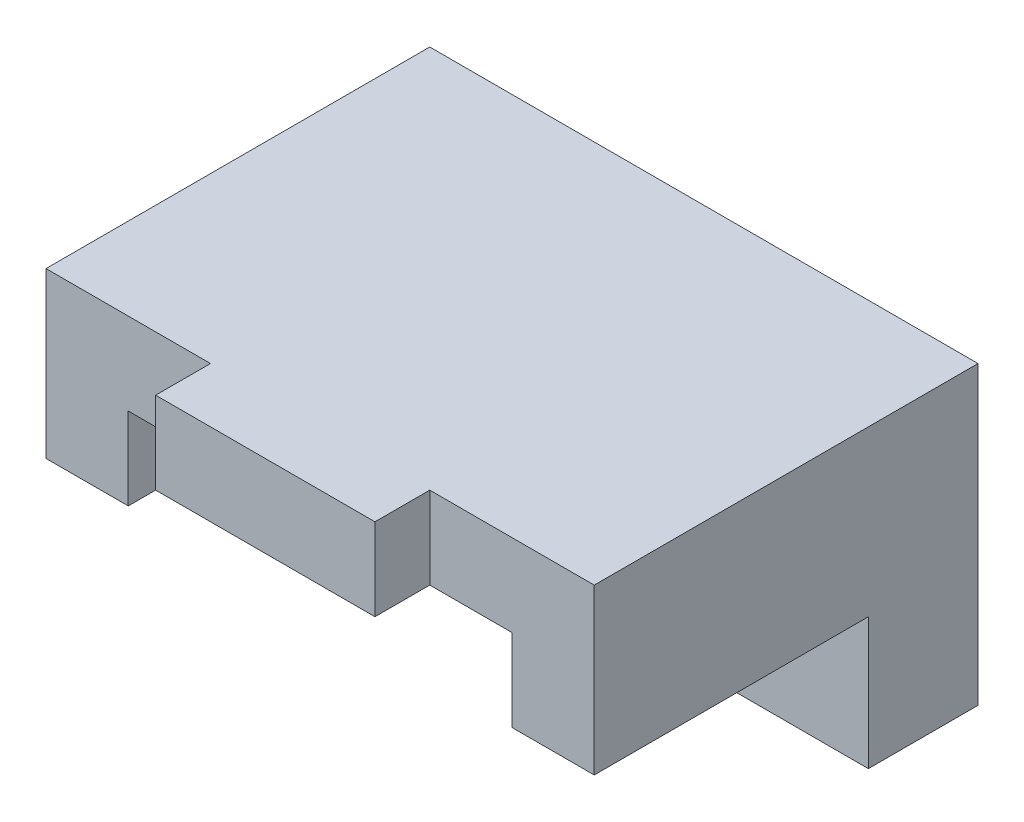
ISO-10303-21;
HEADER;
FILE_DESCRIPTION(('STEP AP214'),'2;1');
FILE_NAME('part.step','',(''),(''),'','','');
FILE_SCHEMA(('AUTOMOTIVE_DESIGN { 1 0 10303 214 1 1 1 1 }'));
ENDSEC;
DATA;
#1=APPLICATION_CONTEXT('core data for automotive mechanical design processes');
#2=APPLICATION_PROTOCOL_DEFINITION('international standard','automotive_design',2000,#1);
#3=PRODUCT_CONTEXT('',#1,'mechanical');
#4=PRODUCT('Part','Part','',(#3));
#5=PRODUCT_RELATED_PRODUCT_CATEGORY('part','',(#4));
#6=PRODUCT_DEFINITION_FORMATION('','',#4);
#7=PRODUCT_DEFINITION_CONTEXT('part definition',#1,'design');
#8=PRODUCT_DEFINITION('design','',#6,#7);
#9=PRODUCT_DEFINITION_SHAPE('','',#8);
#10=(LENGTH_UNIT() NAMED_UNIT(*) SI_UNIT(.MILLI.,.METRE.));
#11=(NAMED_UNIT(*) PLANE_ANGLE_UNIT() SI_UNIT($,.RADIAN.));
#12=(NAMED_UNIT(*) SI_UNIT($,.STERADIAN.) SOLID_ANGLE_UNIT());
#13=UNCERTAINTY_MEASURE_WITH_UNIT(LENGTH_MEASURE(1.E-05),#10,'distance_accuracy_value','');
#14=(GEOMETRIC_REPRESENTATION_CONTEXT(3) GLOBAL_UNCERTAINTY_ASSIGNED_CONTEXT((#13)) GLOBAL_UNIT_ASSIGNED_CONTEXT((#10,
#11,#12)) REPRESENTATION_CONTEXT('',''));
#15=CARTESIAN_POINT('',(0.,0.,0.));
#16=DIRECTION('',(0.,0.,1.));
#17=DIRECTION('',(1.,0.,0.));
#18=AXIS2_PLACEMENT_3D('',#15,#16,#17);
#19=CARTESIAN_POINT('',(0.,0.,200.));
#20=DIRECTION('',(0.,1.,0.));
#21=DIRECTION('',(0.,0.,1.));
#22=AXIS2_PLACEMENT_3D('',#19,#20,#21);
#23=PLANE('',#22);
#24=DIRECTION('',(0.,0.,1.));
#25=VECTOR('',#24,1.);
#26=CARTESIAN_POINT('',(750.,0.,50.));
#27=LINE('',#26,#25);
#28=CARTESIAN_POINT('',(750.,0.,50.));
#29=VERTEX_POINT('',#28);
#30=CARTESIAN_POINT('',(750.,0.,200.));
#31=VERTEX_POINT('',#30);
#32=EDGE_CURVE('E242',#29,#31,#27,.T.);
#33=ORIENTED_EDGE('',*,*,#32,.F.);
#34=DIRECTION('',(1.,0.,0.));
#35=VECTOR('',#34,1.);
#36=CARTESIAN_POINT('',(0.,0.,50.));
#37=LINE('',#36,#35);
#38=CARTESIAN_POINT('',(250.,0.,50.));
#39=VERTEX_POINT('',#38);
#40=EDGE_CURVE('E233',#39,#29,#37,.T.);
#41=ORIENTED_EDGE('',*,*,#40,.F.);
#42=DIRECTION('',(0.,0.,1.));
#43=VECTOR('',#42,1.);
#44=CARTESIAN_POINT('',(250.,0.,50.));
#45=LINE('',#44,#43);
#46=CARTESIAN_POINT('',(250.,0.,200.));
#47=VERTEX_POINT('',#46);
#48=EDGE_CURVE('E246',#39,#47,#45,.T.);
#49=ORIENTED_EDGE('',*,*,#48,.T.);
#50=DIRECTION('',(1.,0.,0.));
#51=VECTOR('',#50,1.);
#52=CARTESIAN_POINT('',(0.,0.,200.));
#53=LINE('',#52,#51);
#54=CARTESIAN_POINT('',(0.,0.,200.));
#55=VERTEX_POINT('',#54);
#56=EDGE_CURVE('E326',#55,#47,#53,.T.);
#57=ORIENTED_EDGE('',*,*,#56,.F.);
#58=DIRECTION('',(0.,0.,-1.));
#59=VECTOR('',#58,1.);
#60=CARTESIAN_POINT('',(0.,0.,200.));
#61=LINE('',#60,#59);
#62=CARTESIAN_POINT('',(0.,0.,0.));
#63=VERTEX_POINT('',#62);
#64=EDGE_CURVE('E11',#55,#63,#61,.T.);
#65=ORIENTED_EDGE('',*,*,#64,.T.);
#66=DIRECTION('',(1.,0.,0.));
#67=VECTOR('',#66,1.);
#68=CARTESIAN_POINT('',(0.,0.,0.));
#69=LINE('',#68,#67);
#70=CARTESIAN_POINT('',(1000.,0.,0.));
#71=VERTEX_POINT('',#70);
#72=EDGE_CURVE('E335',#63,#71,#69,.T.);
#73=ORIENTED_EDGE('',*,*,#72,.T.);
#74=DIRECTION('',(0.,0.,-1.));
#75=VECTOR('',#74,1.);
#76=CARTESIAN_POINT('',(1000.,0.,200.));
#77=LINE('',#76,#75);
#78=CARTESIAN_POINT('',(1000.,0.,200.));
#79=VERTEX_POINT('',#78);
#80=EDGE_CURVE('E54',#79,#71,#77,.T.);
#81=ORIENTED_EDGE('',*,*,#80,.F.);
#82=EDGE_CURVE('E321',#31,#79,#53,.T.);
#83=ORIENTED_EDGE('',*,*,#82,.F.);
#84=EDGE_LOOP('',(#33,#41,#49,#57,#65,#73,#81,#83));
#85=FACE_BOUND('',#84,.T.);
#86=ADVANCED_FACE('F50',(#85),#23,.F.);
#87=CARTESIAN_POINT('',(0.,0.,200.));
#88=DIRECTION('',(0.,0.,1.));
#89=DIRECTION('',(1.,0.,0.));
#90=AXIS2_PLACEMENT_3D('',#87,#88,#89);
#91=PLANE('',#90);
#92=DIRECTION('',(0.,1.,0.));
#93=VECTOR('',#92,1.);
#94=CARTESIAN_POINT('',(250.,0.,200.));
#95=LINE('',#94,#93);
#96=CARTESIAN_POINT('',(250.,240.,200.));
#97=VERTEX_POINT('',#96);
#98=EDGE_CURVE('E221',#47,#97,#95,.T.);
#99=ORIENTED_EDGE('',*,*,#98,.T.);
#100=DIRECTION('',(-1.,0.,0.));
#101=VECTOR('',#100,1.);
#102=CARTESIAN_POINT('',(250.,240.,200.));
#103=LINE('',#102,#101);
#104=CARTESIAN_POINT('',(750.,240.,200.));
#105=VERTEX_POINT('',#104);
#106=EDGE_CURVE('E215',#105,#97,#103,.T.);
#107=ORIENTED_EDGE('',*,*,#106,.F.);
#108=DIRECTION('',(0.,-1.,0.));
#109=VECTOR('',#108,1.);
#110=CARTESIAN_POINT('',(750.,0.,200.));
#111=LINE('',#110,#109);
#112=EDGE_CURVE('E230',#105,#31,#111,.T.);
#113=ORIENTED_EDGE('',*,*,#112,.T.);
#114=ORIENTED_EDGE('',*,*,#82,.T.);
#115=DIRECTION('',(0.,1.,0.));
#116=VECTOR('',#115,1.);
#117=CARTESIAN_POINT('',(1000.,0.,200.));
#118=LINE('',#117,#116);
#119=CARTESIAN_POINT('',(1000.,240.,200.));
#120=VERTEX_POINT('',#119);
#121=EDGE_CURVE('E327',#79,#120,#118,.T.);
#122=ORIENTED_EDGE('',*,*,#121,.T.);
#123=DIRECTION('',(1.,0.,0.));
#124=VECTOR('',#123,1.);
#125=CARTESIAN_POINT('',(0.,240.,200.));
#126=LINE('',#125,#124);
#127=CARTESIAN_POINT('',(850.,240.,200.));
#128=VERTEX_POINT('',#127);
#129=EDGE_CURVE('E314',#128,#120,#126,.T.);
#130=ORIENTED_EDGE('',*,*,#129,.F.);
#131=DIRECTION('',(0.,-1.,0.));
#132=VECTOR('',#131,1.);
#133=CARTESIAN_POINT('',(850.,390.,200.));
#134=LINE('',#133,#132);
#135=CARTESIAN_POINT('',(850.,390.,200.));
#136=VERTEX_POINT('',#135);
#137=EDGE_CURVE('E272',#136,#128,#134,.T.);
#138=ORIENTED_EDGE('',*,*,#137,.F.);
#139=DIRECTION('',(1.,0.,0.));
#140=VECTOR('',#139,1.);
#141=CARTESIAN_POINT('',(150.,390.,200.));
#142=LINE('',#141,#140);
#143=CARTESIAN_POINT('',(150.,390.,200.));
#144=VERTEX_POINT('',#143);
#145=EDGE_CURVE('E260',#144,#136,#142,.T.);
#146=ORIENTED_EDGE('',*,*,#145,.F.);
#147=DIRECTION('',(0.,-1.,0.));
#148=VECTOR('',#147,1.);
#149=CARTESIAN_POINT('',(150.,390.,200.));
#150=LINE('',#149,#148);
#151=CARTESIAN_POINT('',(150.,240.,200.));
#152=VERTEX_POINT('',#151);
#153=EDGE_CURVE('E271',#144,#152,#150,.T.);
#154=ORIENTED_EDGE('',*,*,#153,.T.);
#155=CARTESIAN_POINT('',(0.,240.,200.));
#156=VERTEX_POINT('',#155);
#157=EDGE_CURVE('E319',#156,#152,#126,.T.);
#158=ORIENTED_EDGE('',*,*,#157,.F.);
#159=DIRECTION('',(0.,-1.,0.));
#160=VECTOR('',#159,1.);
#161=CARTESIAN_POINT('',(0.,540.,200.));
#162=LINE('',#161,#160);
#163=EDGE_CURVE('E325',#156,#55,#162,.T.);
#164=ORIENTED_EDGE('',*,*,#163,.T.);
#165=ORIENTED_EDGE('',*,*,#56,.T.);
#166=EDGE_LOOP('',(#99,#107,#113,#114,#122,#130,#138,#146,#154,#158,#164,#165));
#167=FACE_BOUND('',#166,.T.);
#168=ADVANCED_FACE('F371',(#167),#91,.T.);
#169=CARTESIAN_POINT('',(0.,240.,800.));
#170=DIRECTION('',(0.,-1.,0.));
#171=DIRECTION('',(0.,0.,-1.));
#172=AXIS2_PLACEMENT_3D('',#169,#170,#171);
#173=PLANE('',#172);
#174=DIRECTION('',(0.,0.,1.));
#175=VECTOR('',#174,1.);
#176=CARTESIAN_POINT('',(850.,240.,200.));
#177=LINE('',#176,#175);
#178=CARTESIAN_POINT('',(850.,240.,700.));
#179=VERTEX_POINT('',#178);
#180=EDGE_CURVE('E266',#128,#179,#177,.T.);
#181=ORIENTED_EDGE('',*,*,#180,.F.);
#182=ORIENTED_EDGE('',*,*,#129,.T.);
#183=DIRECTION('',(0.,0.,-1.));
#184=VECTOR('',#183,1.);
#185=CARTESIAN_POINT('',(1000.,240.,800.));
#186=LINE('',#185,#184);
#187=CARTESIAN_POINT('',(1000.,240.,700.));
#188=VERTEX_POINT('',#187);
#189=EDGE_CURVE('E315',#188,#120,#186,.T.);
#190=ORIENTED_EDGE('',*,*,#189,.F.);
#191=DIRECTION('',(1.,0.,0.));
#192=VECTOR('',#191,1.);
#193=CARTESIAN_POINT('',(0.,240.,700.));
#194=LINE('',#193,#192);
#195=EDGE_CURVE('E306',#179,#188,#194,.T.);
#196=ORIENTED_EDGE('',*,*,#195,.F.);
#197=EDGE_LOOP('',(#181,#182,#190,#196));
#198=FACE_BOUND('',#197,.T.);
#199=ADVANCED_FACE('F368',(#198),#173,.T.);
#200=CARTESIAN_POINT('',(0.,0.,700.));
#201=DIRECTION('',(0.,0.,1.));
#202=DIRECTION('',(1.,0.,0.));
#203=AXIS2_PLACEMENT_3D('',#200,#201,#202);
#204=PLANE('',#203);
#205=DIRECTION('',(0.,-1.,0.));
#206=VECTOR('',#205,1.);
#207=CARTESIAN_POINT('',(150.,390.,700.));
#208=LINE('',#207,#206);
#209=CARTESIAN_POINT('',(150.,390.,700.));
#210=VERTEX_POINT('',#209);
#211=CARTESIAN_POINT('',(150.,240.,700.));
#212=VERTEX_POINT('',#211);
#213=EDGE_CURVE('E263',#210,#212,#208,.T.);
#214=ORIENTED_EDGE('',*,*,#213,.F.);
#215=DIRECTION('',(-1.,0.,0.));
#216=VECTOR('',#215,1.);
#217=CARTESIAN_POINT('',(850.,390.,700.));
#218=LINE('',#217,#216);
#219=CARTESIAN_POINT('',(300.,390.,700.));
#220=VERTEX_POINT('',#219);
#221=EDGE_CURVE('E251',#220,#210,#218,.T.);
#222=ORIENTED_EDGE('',*,*,#221,.F.);
#223=DIRECTION('',(0.,1.,0.));
#224=VECTOR('',#223,1.);
#225=CARTESIAN_POINT('',(300.,390.,700.));
#226=LINE('',#225,#224);
#227=CARTESIAN_POINT('',(300.,540.,700.));
#228=VERTEX_POINT('',#227);
#229=EDGE_CURVE('E291',#220,#228,#226,.T.);
#230=ORIENTED_EDGE('',*,*,#229,.T.);
#231=DIRECTION('',(-1.,0.,0.));
#232=VECTOR('',#231,1.);
#233=CARTESIAN_POINT('',(1000.,540.,700.));
#234=LINE('',#233,#232);
#235=CARTESIAN_POINT('',(0.,540.,700.));
#236=VERTEX_POINT('',#235);
#237=EDGE_CURVE('E294',#228,#236,#234,.T.);
#238=ORIENTED_EDGE('',*,*,#237,.T.);
#239=DIRECTION('',(0.,-1.,0.));
#240=VECTOR('',#239,1.);
#241=CARTESIAN_POINT('',(0.,540.,700.));
#242=LINE('',#241,#240);
#243=CARTESIAN_POINT('',(0.,240.,700.));
#244=VERTEX_POINT('',#243);
#245=EDGE_CURVE('E302',#236,#244,#242,.T.);
#246=ORIENTED_EDGE('',*,*,#245,.T.);
#247=EDGE_CURVE('E310',#244,#212,#194,.T.);
#248=ORIENTED_EDGE('',*,*,#247,.T.);
#249=EDGE_LOOP('',(#214,#222,#230,#238,#246,#248));
#250=FACE_BOUND('',#249,.T.);
#251=ADVANCED_FACE('F414',(#250),#204,.T.);
#252=CARTESIAN_POINT('',(0.,540.,200.));
#253=DIRECTION('',(1.,0.,0.));
#254=DIRECTION('',(0.,0.,-1.));
#255=AXIS2_PLACEMENT_3D('',#252,#253,#254);
#256=PLANE('',#255);
#257=ORIENTED_EDGE('',*,*,#245,.F.);
#258=DIRECTION('',(0.,0.,-1.));
#259=VECTOR('',#258,1.);
#260=CARTESIAN_POINT('',(0.,540.,200.));
#261=LINE('',#260,#259);
#262=CARTESIAN_POINT('',(0.,540.,0.));
#263=VERTEX_POINT('',#262);
#264=EDGE_CURVE('E332',#236,#263,#261,.T.);
#265=ORIENTED_EDGE('',*,*,#264,.T.);
#266=DIRECTION('',(0.,-1.,0.));
#267=VECTOR('',#266,1.);
#268=CARTESIAN_POINT('',(0.,540.,0.));
#269=LINE('',#268,#267);
#270=EDGE_CURVE('E322',#263,#63,#269,.T.);
#271=ORIENTED_EDGE('',*,*,#270,.T.);
#272=ORIENTED_EDGE('',*,*,#64,.F.);
#273=ORIENTED_EDGE('',*,*,#163,.F.);
#274=DIRECTION('',(0.,0.,-1.));
#275=VECTOR('',#274,1.);
#276=CARTESIAN_POINT('',(0.,240.,800.));
#277=LINE('',#276,#275);
#278=EDGE_CURVE('E312',#244,#156,#277,.T.);
#279=ORIENTED_EDGE('',*,*,#278,.F.);
#280=EDGE_LOOP('',(#257,#265,#271,#272,#273,#279));
#281=FACE_BOUND('',#280,.T.);
#282=ADVANCED_FACE('F47',(#281),#256,.F.);
#283=CARTESIAN_POINT('',(1000.,0.,200.));
#284=DIRECTION('',(-1.,0.,0.));
#285=DIRECTION('',(0.,0.,1.));
#286=AXIS2_PLACEMENT_3D('',#283,#284,#285);
#287=PLANE('',#286);
#288=DIRECTION('',(0.,1.,0.));
#289=VECTOR('',#288,1.);
#290=CARTESIAN_POINT('',(1000.,240.,700.));
#291=LINE('',#290,#289);
#292=CARTESIAN_POINT('',(1000.,540.,700.));
#293=VERTEX_POINT('',#292);
#294=EDGE_CURVE('E309',#188,#293,#291,.T.);
#295=ORIENTED_EDGE('',*,*,#294,.F.);
#296=ORIENTED_EDGE('',*,*,#189,.T.);
#297=ORIENTED_EDGE('',*,*,#121,.F.);
#298=ORIENTED_EDGE('',*,*,#80,.T.);
#299=DIRECTION('',(0.,1.,0.));
#300=VECTOR('',#299,1.);
#301=CARTESIAN_POINT('',(1000.,0.,0.));
#302=LINE('',#301,#300);
#303=CARTESIAN_POINT('',(1000.,540.,0.));
#304=VERTEX_POINT('',#303);
#305=EDGE_CURVE('E340',#71,#304,#302,.T.);
#306=ORIENTED_EDGE('',*,*,#305,.T.);
#307=DIRECTION('',(0.,0.,-1.));
#308=VECTOR('',#307,1.);
#309=CARTESIAN_POINT('',(1000.,540.,200.));
#310=LINE('',#309,#308);
#311=EDGE_CURVE('E344',#293,#304,#310,.T.);
#312=ORIENTED_EDGE('',*,*,#311,.F.);
#313=EDGE_LOOP('',(#295,#296,#297,#298,#306,#312));
#314=FACE_BOUND('',#313,.T.);
#315=ADVANCED_FACE('F349',(#314),#287,.F.);
#316=CARTESIAN_POINT('',(1000.,540.,200.));
#317=DIRECTION('',(0.,-1.,0.));
#318=DIRECTION('',(0.,0.,-1.));
#319=AXIS2_PLACEMENT_3D('',#316,#317,#318);
#320=PLANE('',#319);
#321=CARTESIAN_POINT('',(700.,540.,700.));
#322=VERTEX_POINT('',#321);
#323=EDGE_CURVE('E301',#293,#322,#234,.T.);
#324=ORIENTED_EDGE('',*,*,#323,.F.);
#325=ORIENTED_EDGE('',*,*,#311,.T.);
#326=DIRECTION('',(-1.,0.,0.));
#327=VECTOR('',#326,1.);
#328=CARTESIAN_POINT('',(1000.,540.,0.));
#329=LINE('',#328,#327);
#330=EDGE_CURVE('E323',#304,#263,#329,.T.);
#331=ORIENTED_EDGE('',*,*,#330,.T.);
#332=ORIENTED_EDGE('',*,*,#264,.F.);
#333=ORIENTED_EDGE('',*,*,#237,.F.);
#334=DIRECTION('',(0.,0.,1.));
#335=VECTOR('',#334,1.);
#336=CARTESIAN_POINT('',(300.,540.,0.));
#337=LINE('',#336,#335);
#338=CARTESIAN_POINT('',(300.,540.,800.));
#339=VERTEX_POINT('',#338);
#340=EDGE_CURVE('E69',#228,#339,#337,.T.);
#341=ORIENTED_EDGE('',*,*,#340,.T.);
#342=DIRECTION('',(1.,0.,0.));
#343=VECTOR('',#342,1.);
#344=CARTESIAN_POINT('',(0.,540.,800.));
#345=LINE('',#344,#343);
#346=CARTESIAN_POINT('',(700.,540.,800.));
#347=VERTEX_POINT('',#346);
#348=EDGE_CURVE('E289',#339,#347,#345,.T.);
#349=ORIENTED_EDGE('',*,*,#348,.T.);
#350=DIRECTION('',(0.,0.,-1.));
#351=VECTOR('',#350,1.);
#352=CARTESIAN_POINT('',(700.,540.,0.));
#353=LINE('',#352,#351);
#354=EDGE_CURVE('E278',#347,#322,#353,.T.);
#355=ORIENTED_EDGE('',*,*,#354,.T.);
#356=EDGE_LOOP('',(#324,#325,#331,#332,#333,#341,#349,#355));
#357=FACE_BOUND('',#356,.T.);
#358=ADVANCED_FACE('F363',(#357),#320,.F.);
#359=DIRECTION('',(0.,0.,-1.));
#360=VECTOR('',#359,1.);
#361=CARTESIAN_POINT('',(150.,240.,700.));
#362=LINE('',#361,#360);
#363=EDGE_CURVE('E243',#212,#152,#362,.T.);
#364=ORIENTED_EDGE('',*,*,#363,.F.);
#365=ORIENTED_EDGE('',*,*,#247,.F.);
#366=ORIENTED_EDGE('',*,*,#278,.T.);
#367=ORIENTED_EDGE('',*,*,#157,.T.);
#368=EDGE_LOOP('',(#364,#365,#366,#367));
#369=FACE_BOUND('',#368,.T.);
#370=ADVANCED_FACE('F419',(#369),#173,.T.);
#371=CARTESIAN_POINT('',(0.,0.,0.));
#372=DIRECTION('',(0.,0.,1.));
#373=DIRECTION('',(1.,0.,0.));
#374=AXIS2_PLACEMENT_3D('',#371,#372,#373);
#375=PLANE('',#374);
#376=ORIENTED_EDGE('',*,*,#270,.F.);
#377=ORIENTED_EDGE('',*,*,#330,.F.);
#378=ORIENTED_EDGE('',*,*,#305,.F.);
#379=ORIENTED_EDGE('',*,*,#72,.F.);
#380=EDGE_LOOP('',(#376,#377,#378,#379));
#381=FACE_BOUND('',#380,.T.);
#382=ADVANCED_FACE('F357',(#381),#375,.F.);
#383=DIRECTION('',(0.,-1.,0.));
#384=VECTOR('',#383,1.);
#385=CARTESIAN_POINT('',(850.,390.,700.));
#386=LINE('',#385,#384);
#387=CARTESIAN_POINT('',(850.,390.,700.));
#388=VERTEX_POINT('',#387);
#389=EDGE_CURVE('E269',#388,#179,#386,.T.);
#390=ORIENTED_EDGE('',*,*,#389,.T.);
#391=ORIENTED_EDGE('',*,*,#195,.T.);
#392=ORIENTED_EDGE('',*,*,#294,.T.);
#393=ORIENTED_EDGE('',*,*,#323,.T.);
#394=DIRECTION('',(0.,1.,0.));
#395=VECTOR('',#394,1.);
#396=CARTESIAN_POINT('',(700.,390.,700.));
#397=LINE('',#396,#395);
#398=CARTESIAN_POINT('',(700.,390.,700.));
#399=VERTEX_POINT('',#398);
#400=EDGE_CURVE('E298',#399,#322,#397,.T.);
#401=ORIENTED_EDGE('',*,*,#400,.F.);
#402=EDGE_CURVE('E252',#388,#399,#218,.T.);
#403=ORIENTED_EDGE('',*,*,#402,.F.);
#404=EDGE_LOOP('',(#390,#391,#392,#393,#401,#403));
#405=FACE_BOUND('',#404,.T.);
#406=ADVANCED_FACE('F434',(#405),#204,.T.);
#407=CARTESIAN_POINT('',(300.,390.,0.));
#408=DIRECTION('',(-1.,0.,0.));
#409=DIRECTION('',(0.,0.,1.));
#410=AXIS2_PLACEMENT_3D('',#407,#408,#409);
#411=PLANE('',#410);
#412=ORIENTED_EDGE('',*,*,#340,.F.);
#413=ORIENTED_EDGE('',*,*,#229,.F.);
#414=DIRECTION('',(0.,0.,1.));
#415=VECTOR('',#414,1.);
#416=CARTESIAN_POINT('',(300.,390.,0.));
#417=LINE('',#416,#415);
#418=CARTESIAN_POINT('',(300.,390.,800.));
#419=VERTEX_POINT('',#418);
#420=EDGE_CURVE('E277',#220,#419,#417,.T.);
#421=ORIENTED_EDGE('',*,*,#420,.T.);
#422=DIRECTION('',(0.,1.,0.));
#423=VECTOR('',#422,1.);
#424=CARTESIAN_POINT('',(300.,390.,800.));
#425=LINE('',#424,#423);
#426=EDGE_CURVE('E286',#419,#339,#425,.T.);
#427=ORIENTED_EDGE('',*,*,#426,.T.);
#428=EDGE_LOOP('',(#412,#413,#421,#427));
#429=FACE_BOUND('',#428,.T.);
#430=ADVANCED_FACE('F424',(#429),#411,.T.);
#431=CARTESIAN_POINT('',(700.,390.,0.));
#432=DIRECTION('',(1.,0.,0.));
#433=DIRECTION('',(0.,0.,-1.));
#434=AXIS2_PLACEMENT_3D('',#431,#432,#433);
#435=PLANE('',#434);
#436=ORIENTED_EDGE('',*,*,#354,.F.);
#437=DIRECTION('',(0.,1.,0.));
#438=VECTOR('',#437,1.);
#439=CARTESIAN_POINT('',(700.,390.,800.));
#440=LINE('',#439,#438);
#441=CARTESIAN_POINT('',(700.,390.,800.));
#442=VERTEX_POINT('',#441);
#443=EDGE_CURVE('E296',#442,#347,#440,.T.);
#444=ORIENTED_EDGE('',*,*,#443,.F.);
#445=DIRECTION('',(0.,0.,-1.));
#446=VECTOR('',#445,1.);
#447=CARTESIAN_POINT('',(700.,390.,0.));
#448=LINE('',#447,#446);
#449=EDGE_CURVE('E283',#442,#399,#448,.T.);
#450=ORIENTED_EDGE('',*,*,#449,.T.);
#451=ORIENTED_EDGE('',*,*,#400,.T.);
#452=EDGE_LOOP('',(#436,#444,#450,#451));
#453=FACE_BOUND('',#452,.T.);
#454=ADVANCED_FACE('F440',(#453),#435,.T.);
#455=CARTESIAN_POINT('',(0.,390.,800.));
#456=DIRECTION('',(0.,0.,1.));
#457=DIRECTION('',(1.,0.,0.));
#458=AXIS2_PLACEMENT_3D('',#455,#456,#457);
#459=PLANE('',#458);
#460=ORIENTED_EDGE('',*,*,#348,.F.);
#461=ORIENTED_EDGE('',*,*,#426,.F.);
#462=DIRECTION('',(1.,0.,0.));
#463=VECTOR('',#462,1.);
#464=CARTESIAN_POINT('',(0.,390.,800.));
#465=LINE('',#464,#463);
#466=EDGE_CURVE('E276',#419,#442,#465,.T.);
#467=ORIENTED_EDGE('',*,*,#466,.T.);
#468=ORIENTED_EDGE('',*,*,#443,.T.);
#469=EDGE_LOOP('',(#460,#461,#467,#468));
#470=FACE_BOUND('',#469,.T.);
#471=ADVANCED_FACE('F431',(#470),#459,.T.);
#472=CARTESIAN_POINT('',(0.,390.,0.));
#473=DIRECTION('',(0.,1.,0.));
#474=DIRECTION('',(0.,0.,1.));
#475=AXIS2_PLACEMENT_3D('',#472,#473,#474);
#476=PLANE('',#475);
#477=ORIENTED_EDGE('',*,*,#420,.F.);
#478=ORIENTED_EDGE('',*,*,#221,.T.);
#479=DIRECTION('',(0.,0.,-1.));
#480=VECTOR('',#479,1.);
#481=CARTESIAN_POINT('',(150.,390.,700.));
#482=LINE('',#481,#480);
#483=EDGE_CURVE('E254',#210,#144,#482,.T.);
#484=ORIENTED_EDGE('',*,*,#483,.T.);
#485=ORIENTED_EDGE('',*,*,#145,.T.);
#486=DIRECTION('',(0.,0.,1.));
#487=VECTOR('',#486,1.);
#488=CARTESIAN_POINT('',(850.,390.,200.));
#489=LINE('',#488,#487);
#490=EDGE_CURVE('E258',#136,#388,#489,.T.);
#491=ORIENTED_EDGE('',*,*,#490,.T.);
#492=ORIENTED_EDGE('',*,*,#402,.T.);
#493=ORIENTED_EDGE('',*,*,#449,.F.);
#494=ORIENTED_EDGE('',*,*,#466,.F.);
#495=EDGE_LOOP('',(#477,#478,#484,#485,#491,#492,#493,#494));
#496=FACE_BOUND('',#495,.T.);
#497=ADVANCED_FACE('F430',(#496),#476,.F.);
#498=CARTESIAN_POINT('',(850.,390.,200.));
#499=DIRECTION('',(1.,0.,0.));
#500=DIRECTION('',(0.,0.,-1.));
#501=AXIS2_PLACEMENT_3D('',#498,#499,#500);
#502=PLANE('',#501);
#503=ORIENTED_EDGE('',*,*,#180,.T.);
#504=ORIENTED_EDGE('',*,*,#389,.F.);
#505=ORIENTED_EDGE('',*,*,#490,.F.);
#506=ORIENTED_EDGE('',*,*,#137,.T.);
#507=EDGE_LOOP('',(#503,#504,#505,#506));
#508=FACE_BOUND('',#507,.T.);
#509=ADVANCED_FACE('F539',(#508),#502,.F.);
#510=CARTESIAN_POINT('',(150.,390.,700.));
#511=DIRECTION('',(-1.,0.,0.));
#512=DIRECTION('',(0.,0.,1.));
#513=AXIS2_PLACEMENT_3D('',#510,#511,#512);
#514=PLANE('',#513);
#515=ORIENTED_EDGE('',*,*,#363,.T.);
#516=ORIENTED_EDGE('',*,*,#153,.F.);
#517=ORIENTED_EDGE('',*,*,#483,.F.);
#518=ORIENTED_EDGE('',*,*,#213,.T.);
#519=EDGE_LOOP('',(#515,#516,#517,#518));
#520=FACE_BOUND('',#519,.T.);
#521=ADVANCED_FACE('F423',(#520),#514,.F.);
#522=CARTESIAN_POINT('',(0.,80.,50.));
#523=DIRECTION('',(0.,-1.,0.));
#524=DIRECTION('',(0.,0.,-1.));
#525=AXIS2_PLACEMENT_3D('',#522,#523,#524);
#526=PLANE('',#525);
#527=DIRECTION('',(1.,0.,0.));
#528=VECTOR('',#527,1.);
#529=CARTESIAN_POINT('',(750.,80.,100.));
#530=LINE('',#529,#528);
#531=CARTESIAN_POINT('',(250.,80.,100.));
#532=VERTEX_POINT('',#531);
#533=CARTESIAN_POINT('',(750.,80.,100.));
#534=VERTEX_POINT('',#533);
#535=EDGE_CURVE('E386',#532,#534,#530,.T.);
#536=ORIENTED_EDGE('',*,*,#535,.F.);
#537=DIRECTION('',(0.,0.,1.));
#538=VECTOR('',#537,1.);
#539=CARTESIAN_POINT('',(250.,80.,50.));
#540=LINE('',#539,#538);
#541=CARTESIAN_POINT('',(250.,80.,50.));
#542=VERTEX_POINT('',#541);
#543=EDGE_CURVE('E236',#542,#532,#540,.T.);
#544=ORIENTED_EDGE('',*,*,#543,.F.);
#545=DIRECTION('',(1.,0.,0.));
#546=VECTOR('',#545,1.);
#547=CARTESIAN_POINT('',(0.,80.,50.));
#548=LINE('',#547,#546);
#549=CARTESIAN_POINT('',(750.,80.,50.));
#550=VERTEX_POINT('',#549);
#551=EDGE_CURVE('E225',#542,#550,#548,.T.);
#552=ORIENTED_EDGE('',*,*,#551,.T.);
#553=DIRECTION('',(0.,0.,1.));
#554=VECTOR('',#553,1.);
#555=CARTESIAN_POINT('',(750.,80.,50.));
#556=LINE('',#555,#554);
#557=EDGE_CURVE('E239',#550,#534,#556,.T.);
#558=ORIENTED_EDGE('',*,*,#557,.T.);
#559=EDGE_LOOP('',(#536,#544,#552,#558));
#560=FACE_BOUND('',#559,.T.);
#561=ADVANCED_FACE('F390',(#560),#526,.T.);
#562=CARTESIAN_POINT('',(750.,0.,50.));
#563=DIRECTION('',(-1.,0.,0.));
#564=DIRECTION('',(0.,0.,1.));
#565=AXIS2_PLACEMENT_3D('',#562,#563,#564);
#566=PLANE('',#565);
#567=ORIENTED_EDGE('',*,*,#112,.F.);
#568=DIRECTION('',(0.,0.,1.));
#569=VECTOR('',#568,1.);
#570=CARTESIAN_POINT('',(750.,240.,150.));
#571=LINE('',#570,#569);
#572=CARTESIAN_POINT('',(750.,240.,150.));
#573=VERTEX_POINT('',#572);
#574=EDGE_CURVE('E203',#573,#105,#571,.T.);
#575=ORIENTED_EDGE('',*,*,#574,.F.);
#576=DIRECTION('',(0.,1.,0.));
#577=VECTOR('',#576,1.);
#578=CARTESIAN_POINT('',(750.,240.,150.));
#579=LINE('',#578,#577);
#580=CARTESIAN_POINT('',(750.,160.,150.));
#581=VERTEX_POINT('',#580);
#582=EDGE_CURVE('E198',#581,#573,#579,.T.);
#583=ORIENTED_EDGE('',*,*,#582,.F.);
#584=DIRECTION('',(0.,0.,1.));
#585=VECTOR('',#584,1.);
#586=CARTESIAN_POINT('',(750.,160.,100.));
#587=LINE('',#586,#585);
#588=CARTESIAN_POINT('',(750.,160.,100.));
#589=VERTEX_POINT('',#588);
#590=EDGE_CURVE('E201',#589,#581,#587,.T.);
#591=ORIENTED_EDGE('',*,*,#590,.F.);
#592=DIRECTION('',(0.,1.,0.));
#593=VECTOR('',#592,1.);
#594=CARTESIAN_POINT('',(750.,160.,100.));
#595=LINE('',#594,#593);
#596=EDGE_CURVE('E391',#534,#589,#595,.T.);
#597=ORIENTED_EDGE('',*,*,#596,.F.);
#598=ORIENTED_EDGE('',*,*,#557,.F.);
#599=DIRECTION('',(0.,-1.,0.));
#600=VECTOR('',#599,1.);
#601=CARTESIAN_POINT('',(750.,0.,50.));
#602=LINE('',#601,#600);
#603=EDGE_CURVE('E234',#550,#29,#602,.T.);
#604=ORIENTED_EDGE('',*,*,#603,.T.);
#605=ORIENTED_EDGE('',*,*,#32,.T.);
#606=EDGE_LOOP('',(#567,#575,#583,#591,#597,#598,#604,#605));
#607=FACE_BOUND('',#606,.T.);
#608=ADVANCED_FACE('F197',(#607),#566,.T.);
#609=CARTESIAN_POINT('',(250.,0.,50.));
#610=DIRECTION('',(1.,0.,0.));
#611=DIRECTION('',(0.,0.,-1.));
#612=AXIS2_PLACEMENT_3D('',#609,#610,#611);
#613=PLANE('',#612);
#614=ORIENTED_EDGE('',*,*,#98,.F.);
#615=ORIENTED_EDGE('',*,*,#48,.F.);
#616=DIRECTION('',(0.,1.,0.));
#617=VECTOR('',#616,1.);
#618=CARTESIAN_POINT('',(250.,0.,50.));
#619=LINE('',#618,#617);
#620=EDGE_CURVE('E226',#39,#542,#619,.T.);
#621=ORIENTED_EDGE('',*,*,#620,.T.);
#622=ORIENTED_EDGE('',*,*,#543,.T.);
#623=DIRECTION('',(0.,-1.,0.));
#624=VECTOR('',#623,1.);
#625=CARTESIAN_POINT('',(250.,80.,100.));
#626=LINE('',#625,#624);
#627=CARTESIAN_POINT('',(250.,160.,100.));
#628=VERTEX_POINT('',#627);
#629=EDGE_CURVE('E217',#628,#532,#626,.T.);
#630=ORIENTED_EDGE('',*,*,#629,.F.);
#631=DIRECTION('',(0.,0.,1.));
#632=VECTOR('',#631,1.);
#633=CARTESIAN_POINT('',(250.,160.,100.));
#634=LINE('',#633,#632);
#635=CARTESIAN_POINT('',(250.,160.,150.));
#636=VERTEX_POINT('',#635);
#637=EDGE_CURVE('E218',#628,#636,#634,.T.);
#638=ORIENTED_EDGE('',*,*,#637,.T.);
#639=DIRECTION('',(0.,-1.,0.));
#640=VECTOR('',#639,1.);
#641=CARTESIAN_POINT('',(250.,160.,150.));
#642=LINE('',#641,#640);
#643=CARTESIAN_POINT('',(250.,240.,150.));
#644=VERTEX_POINT('',#643);
#645=EDGE_CURVE('E65',#644,#636,#642,.T.);
#646=ORIENTED_EDGE('',*,*,#645,.F.);
#647=DIRECTION('',(0.,0.,1.));
#648=VECTOR('',#647,1.);
#649=CARTESIAN_POINT('',(250.,240.,150.));
#650=LINE('',#649,#648);
#651=EDGE_CURVE('E395',#644,#97,#650,.T.);
#652=ORIENTED_EDGE('',*,*,#651,.T.);
#653=EDGE_LOOP('',(#614,#615,#621,#622,#630,#638,#646,#652));
#654=FACE_BOUND('',#653,.T.);
#655=ADVANCED_FACE('F384',(#654),#613,.T.);
#656=CARTESIAN_POINT('',(0.,0.,50.));
#657=DIRECTION('',(0.,0.,1.));
#658=DIRECTION('',(1.,0.,0.));
#659=AXIS2_PLACEMENT_3D('',#656,#657,#658);
#660=PLANE('',#659);
#661=ORIENTED_EDGE('',*,*,#551,.F.);
#662=ORIENTED_EDGE('',*,*,#620,.F.);
#663=ORIENTED_EDGE('',*,*,#40,.T.);
#664=ORIENTED_EDGE('',*,*,#603,.F.);
#665=EDGE_LOOP('',(#661,#662,#663,#664));
#666=FACE_BOUND('',#665,.T.);
#667=ADVANCED_FACE('F379',(#666),#660,.T.);
#668=CARTESIAN_POINT('',(250.,160.,100.));
#669=DIRECTION('',(0.,1.,0.));
#670=DIRECTION('',(0.,0.,1.));
#671=AXIS2_PLACEMENT_3D('',#668,#669,#670);
#672=PLANE('',#671);
#673=ORIENTED_EDGE('',*,*,#590,.T.);
#674=DIRECTION('',(1.,0.,0.));
#675=VECTOR('',#674,1.);
#676=CARTESIAN_POINT('',(750.,160.,150.));
#677=LINE('',#676,#675);
#678=EDGE_CURVE('E210',#636,#581,#677,.T.);
#679=ORIENTED_EDGE('',*,*,#678,.F.);
#680=ORIENTED_EDGE('',*,*,#637,.F.);
#681=DIRECTION('',(-1.,0.,0.));
#682=VECTOR('',#681,1.);
#683=CARTESIAN_POINT('',(250.,160.,100.));
#684=LINE('',#683,#682);
#685=EDGE_CURVE('E216',#589,#628,#684,.T.);
#686=ORIENTED_EDGE('',*,*,#685,.F.);
#687=EDGE_LOOP('',(#673,#679,#680,#686));
#688=FACE_BOUND('',#687,.T.);
#689=ADVANCED_FACE('F211',(#688),#672,.F.);
#690=CARTESIAN_POINT('',(0.,0.,100.));
#691=DIRECTION('',(0.,0.,-1.));
#692=DIRECTION('',(-1.,0.,0.));
#693=AXIS2_PLACEMENT_3D('',#690,#691,#692);
#694=PLANE('',#693);
#695=ORIENTED_EDGE('',*,*,#535,.T.);
#696=ORIENTED_EDGE('',*,*,#596,.T.);
#697=ORIENTED_EDGE('',*,*,#685,.T.);
#698=ORIENTED_EDGE('',*,*,#629,.T.);
#699=EDGE_LOOP('',(#695,#696,#697,#698));
#700=FACE_BOUND('',#699,.T.);
#701=ADVANCED_FACE('F398',(#700),#694,.F.);
#702=CARTESIAN_POINT('',(250.,240.,150.));
#703=DIRECTION('',(0.,1.,0.));
#704=DIRECTION('',(0.,0.,1.));
#705=AXIS2_PLACEMENT_3D('',#702,#703,#704);
#706=PLANE('',#705);
#707=ORIENTED_EDGE('',*,*,#106,.T.);
#708=ORIENTED_EDGE('',*,*,#651,.F.);
#709=DIRECTION('',(-1.,0.,0.));
#710=VECTOR('',#709,1.);
#711=CARTESIAN_POINT('',(250.,240.,150.));
#712=LINE('',#711,#710);
#713=EDGE_CURVE('E207',#573,#644,#712,.T.);
#714=ORIENTED_EDGE('',*,*,#713,.F.);
#715=ORIENTED_EDGE('',*,*,#574,.T.);
#716=EDGE_LOOP('',(#707,#708,#714,#715));
#717=FACE_BOUND('',#716,.T.);
#718=ADVANCED_FACE('F403',(#717),#706,.F.);
#719=CARTESIAN_POINT('',(0.,0.,150.));
#720=DIRECTION('',(0.,0.,-1.));
#721=DIRECTION('',(-1.,0.,0.));
#722=AXIS2_PLACEMENT_3D('',#719,#720,#721);
#723=PLANE('',#722);
#724=ORIENTED_EDGE('',*,*,#678,.T.);
#725=ORIENTED_EDGE('',*,*,#582,.T.);
#726=ORIENTED_EDGE('',*,*,#713,.T.);
#727=ORIENTED_EDGE('',*,*,#645,.T.);
#728=EDGE_LOOP('',(#724,#725,#726,#727));
#729=FACE_BOUND('',#728,.T.);
#730=ADVANCED_FACE('F209',(#729),#723,.F.);
#731=CLOSED_SHELL('',(#86,#168,#199,#251,#282,#315,#358,#370,#382,#406,#430,#454,#471,#497,#509,
#521,#561,#608,#655,#667,#689,#701,#718,#730));
#732=MANIFOLD_SOLID_BREP('B2',#731);
#733=ADVANCED_BREP_SHAPE_REPRESENTATION('',(#18,#732),#14);
#734=SHAPE_DEFINITION_REPRESENTATION(#9,#733);
ENDSEC;
END-ISO-10303-21;
